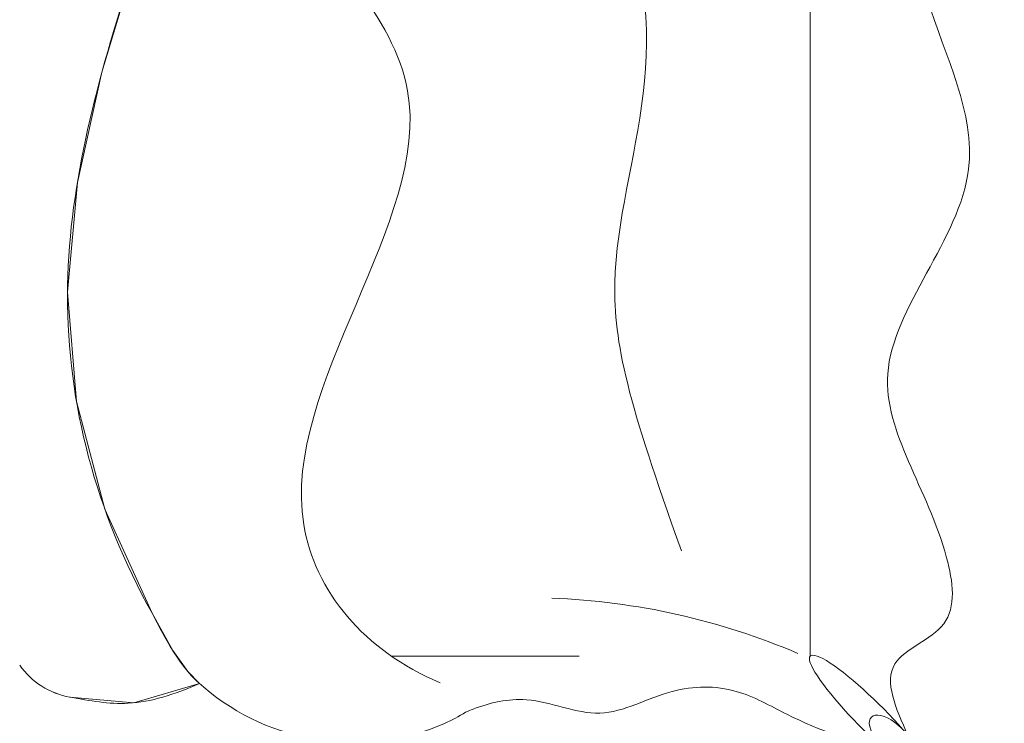
# Model space of a CAD drawing. Units: inches. Extents: x 2083 to 3317, y 1141 to 2115.
# Tile 9 of 256: x 2278 to 2324, y 1296 to 1329. Entities that reach past the tile are written whole.
import ezdxf

# ---------------------------------------------------------------- set-up
doc = ezdxf.new("R2010")
doc.units = ezdxf.units.IN
for name, color, linetype, lineweight in [('A-ANNO-DIMS', 2, 'Continuous', 18), ('A-FURN', 8, 'Continuous', 18), ('www.cadblocksfree.com', 7, 'Continuous', 9)]:
    doc.layers.add(name, color=color, linetype=linetype, lineweight=lineweight)
doc.layers.add('A-WALL-PATT', color=251, linetype='Continuous', lineweight=13, true_color=0x636466)
doc.styles.get("Standard").update_dxf_attribs({"font": 'arial.ttf'})
doc.dimstyles.new('ISO-25', dxfattribs={"dimtxt": 12, "dimasz": 12, "dimexe": 1.25, "dimexo": 0.625, "dimtad": 1, "dimlunit": 3, "dimtxsty": 'Standard', "dimcen": 2.5, "dimadec": 0, "dimazin": 0, "dimtfac": 1, "dimtmove": 0, "dimatfit": 3, "dimfxl": 1, "dimarcsym": 0})

# ---------------------------------------------------------------- blocks, each defined once
blk = doc.blocks.new('bed')
at = {"layer": 'www.cadblocksfree.com', "ltscale": 0.2}
for p, q in [((3363.387, 1412.3), (3363.387, 1402.937)), ((3363.387, 1391.414), (3426.379, 1391.414))]:
    blk.add_line(p, q, dxfattribs=at)
for centre, radius, start, end in [((3365.21, 1427.605), 3.937, 125.4209, 169.6982), ((3370.55, 1414.186), 11.465, 139.4648, 203.3712), ((3367.278, 1412.869), 7.939, 204.0179, 212.619), ((3331.909, 1405.558), 34.378, 336.8495, 357.9003)]:
    blk.add_arc(centre, radius, start, end, dxfattribs=at)
at = {"layer": 'www.cadblocksfree.com', "ltscale": 0.2, "extrusion": (0, 0, -1)}
for centre, major_axis, ratio, start_param, end_param in [((3360.344, 1388.371), (3.043, 3.043), 0.168252, 4.250342, 8.316029), ((3359.289, 1387.316), (1.055, 1.055), 0.453532, 4.422107, 8.144264)]:
    blk.add_ellipse(centre, major_axis=major_axis, ratio=ratio, start_param=start_param, end_param=end_param, dxfattribs=at)
at = {"layer": 'www.cadblocksfree.com', "ltscale": 0.2}
for points, knots in [([(3365.512, 1424.213), (3370.519, 1427.004), (3381.149, 1429.825), (3396.214, 1425.866), (3410.541, 1420.654), (3420.273, 1432.695), (3425.882, 1426.771), (3428.534, 1423.97)], [0.099185, 0.099185, 0.099185, 0.099185, 0.523647, 0.927087, 1.289918, 1.564439, 1.810555, 1.810555, 1.810555, 1.810555]), ([(3361.336, 1428.309), (3361.334, 1428.297), (3361.16, 1427.338), (3360.778, 1425.173), (3361.469, 1423.14), (3362.014, 1421.845)], [0.3128349, 0.3128349, 0.3128349, 0.3128349, 0.313751, 0.386958, 0.4759027, 0.4759027, 0.4759027, 0.4759027]), ([(3362.057, 1409.866), (3363.638, 1413.65), (3372.978, 1421.337), (3389.682, 1406.045), (3402.396, 1419.984), (3416.037, 1420.167), (3423.233, 1415.231), (3427.827, 1408.899)], [0.029901, 0.029901, 0.029901, 0.029901, 0.276967, 0.797115, 1.093669, 1.464666, 1.788489, 1.788489, 1.788489, 1.788489]), ([(3368.632, 1397.839), (3375.978, 1400.489), (3385.349, 1402.757), (3397.531, 1395.273), (3413.593, 1410.377), (3407.806, 1395.019), (3420.759, 1398.2)], [0.029901, 0.029901, 0.029901, 0.029901, 0.276967, 0.797115, 1.093669, 1.16836, 1.16836, 1.16836, 1.16836]), ([(3358.529, 1387.473), (3359.098, 1389.205), (3359.955, 1391.816), (3361.924, 1395.149), (3361.896, 1398.555), (3359.883, 1401.841), (3361.557, 1405.208), (3361.034, 1407.507), (3360.643, 1408.467), (3360.591, 1408.59)], [0, 0, 0, 0, 0.138875, 0.2092702, 0.2901949, 0.3858479, 0.4804923, 0.5489252, 0.5590752, 0.5590752, 0.5590752, 0.5590752]), ([(3430.32, 1386.556), (3427.327, 1387.653), (3422.148, 1389.55), (3414.529, 1384.137), (3405.607, 1387.046), (3396.29, 1386.314), (3386.838, 1381.282), (3377.742, 1390.272), (3370.778, 1384.799), (3364.626, 1383.966), (3363.275, 1388.265), (3360.778, 1387.151), (3359.446, 1386.556)], [0, 0, 0, 0, 8.93042, 15.449194, 25.485629, 34.878505, 43.598887, 54.554403, 64.16647, 67.461673, 70.610457, 74.213583, 74.213583, 74.213583, 74.213583])]:
    blk.add_open_spline(points, degree=3, knots=knots, dxfattribs=at)
for points in [[(3361.235, 1424.042), (3361.236, 1424.042), (3361.237, 1424.043), (3361.239, 1424.043)], [(3361.837, 1421.637), (3362.352, 1422.25), (3362.867, 1422.863), (3365.512, 1424.213)]]:
    blk.add_open_spline(points, degree=3, dxfattribs=at)
blk = doc.blocks.new('*D23')
at = {"layer": 'A-ANNO-DIMS', "color": 0, "lineweight": -2, "transparency": 16777216}
for p, q in [((2335.205, 1362.114), (2335.205, 1476.472)), ((2322.885, 1362.114), (2336.455, 1362.114)), ((2335.205, 1306.473), (2335.205, 1350.114)), ((2322.885, 1294.473), (2336.455, 1294.473))]:
    blk.add_line(p, q, dxfattribs=at)
at = {"layer": 'A-ANNO-DIMS', "color": 0, "transparency": 16777216}
for points in [[(2333.205, 1350.114), (2337.205, 1350.114), (2335.205, 1362.114)], [(2333.205, 1306.473), (2337.205, 1306.473), (2335.205, 1294.473)]]:
    blk.add_solid(points, dxfattribs=at)
at = {"layer": 'Defpoints', "color": 0, "transparency": 16777216}
for p in [(2322.26, 1362.114), (2335.205, 1362.114), (2322.26, 1294.473)]:
    blk.add_point(p, dxfattribs=at)
at = {"layer": 'A-ANNO-DIMS', "color": 0, "transparency": 16777216, "insert": (2328.376, 1425.293), "char_height": 12, "attachment_point": 5, "rotation": 90}
blk.add_mtext('5\'-7 1/2" TYP.', dxfattribs=at)

msp = doc.modelspace()

# ---------------------------------------------------------------- hatches: boundary and pattern name
at = {"layer": 'A-WALL-PATT'}
h = msp.add_hatch(color=256, dxfattribs=at)
h.dxf.hatch_style = 1
h.paths.add_polyline_path([(3126.96, 2020.761), (2748.96, 2020.761), (2604.96, 2020.761), (2226.96, 2020.761), (2226.96, 1702.761), (2466.96, 1702.761), (2466.96, 1582.761), (2418.96, 1582.761), (2418.96, 1477.761), (2226.96, 1477.761), (2226.96, 1263.261), (2544.96, 1263.261), (2544.96, 1411.761), (2604.96, 1411.761), (2685.96, 1411.761), (2685.96, 1420.761), (2604.96, 1420.761), (2604.96, 1573.761), (2604.96, 1702.761), (2604.96, 2011.761), (2748.96, 2011.761), (2748.96, 1702.761), (2862.96, 1702.761), (2862.96, 1621.761), (2871.96, 1621.761), (2871.96, 1702.761), (2883.96, 1702.761), (2883.96, 1706.939, -0.026459), (2883.96, 1711.761), (2757.96, 1711.761), (2757.96, 1807.761), (2787.96, 1807.761), (2787.96, 1812.261), (2757.96, 1812.261), (2757.96, 2011.761), (2877.96, 2011.761), (2877.96, 1812.261), (2847.96, 1812.261), (2847.96, 1807.761), (2889.836, 1807.761), (2889.836, 1812.261), (2882.46, 1812.261), (2882.46, 2011.761), (3117.96, 2011.761), (3117.96, 1812.261), (2937.836, 1812.261), (2937.836, 1807.761), (2995.71, 1807.761), (2995.71, 1796.118), (3000.21, 1796.118), (3000.21, 1807.761), (3117.96, 1807.761), (3117.96, 1711.761), (3000.21, 1711.761), (3000.21, 1760.118), (2998.573, 1760.118, -0.020711), (2995.71, 1760.118), (2995.71, 1711.761), (2931.96, 1711.761), (2931.96, 1702.761), (3126.96, 1702.761)])
h.paths.add_polyline_path([(2471.46, 2011.761), (2471.46, 1810.011), (2462.717, 1810.011), (2462.717, 1805.511), (2505.96, 1805.511), (2505.96, 1810.011), (2475.96, 1810.011), (2475.96, 2011.761), (2595.96, 2011.761), (2595.96, 1810.011), (2565.96, 1810.011), (2565.96, 1805.511), (2595.96, 1805.511), (2595.96, 1711.761), (2235.96, 1711.761), (2235.96, 1805.511), (2353.71, 1805.511), (2353.71, 1796.054), (2358.21, 1796.054), (2358.21, 1805.511), (2414.717, 1805.511), (2414.717, 1810.011), (2235.96, 1810.011), (2235.96, 2011.761)], flags=16)
h.paths.add_polyline_path([(2270.205, 1994.61), (2270.205, 1970.61), (2246.205, 1970.61), (2246.205, 1994.61)], flags=0)
edge = h.paths.add_edge_path(flags=0)
edge.add_ellipse((2332.027, 1899.798), major_axis=(-3.043, 3.043), ratio=0.168252, start_angle=-161.3322, end_angle=-156.3071, ccw=False)
edge.add_ellipse((2333.082, 1898.744), major_axis=(-1.055, 1.055), ratio=0.453532, start_angle=-123.371, end_angle=-94.1591)
edge = h.paths.add_edge_path(flags=0)
edge.add_ellipse((2332.027, 1968.876), major_axis=(3.043, 3.043), ratio=0.168252, start_angle=18.6678, end_angle=23.6929)
edge.add_spline(control_points=[(2332.926, 1970.691), (2332.227, 1970.336), (2330.894, 1969.659), (2328.413, 1970.932), (2327.204, 1967.749), (2324.71, 1969.956), (2322.533, 1967.012), (2320.013, 1971.296), (2317.68, 1968.158), (2316.041, 1967.102), (2315.427, 1966.81)], knot_values=[0, 0, 0, 0, 2.267059, 4.324559, 6.685584, 8.878641, 11.121502, 14.300359, 17.755284, 19.732645, 19.732645, 19.732645, 19.732645], degree=3, periodic=0)
edge.add_ellipse((2332.027, 1968.876), major_axis=(3.043, 3.043), ratio=0.168252, start_angle=18.6678, end_angle=23.6929, ccw=False)
edge.add_ellipse((2333.082, 1969.931), major_axis=(1.055, 1.055), ratio=0.453532, start_angle=56.629, end_angle=85.8409, ccw=False)
edge = h.paths.add_edge_path(flags=0)
edge.add_spline(control_points=[(2296.428, 1967.988), (2293.628, 1965.336), (2287.704, 1959.727), (2299.744, 1949.996), (2294.533, 1935.669), (2290.573, 1920.604), (2293.394, 1909.974), (2296.185, 1904.967)], knot_values=[0.099185, 0.099185, 0.099185, 0.099185, 0.345301, 0.619822, 0.982653, 1.386093, 1.810555, 1.810555, 1.810555, 1.810555], degree=3, periodic=0)
edge.add_spline(control_points=[(2296.185, 1904.967), (2297.384, 1902.619), (2298.001, 1901.949), (2298.553, 1901.468)], knot_values=[0.006246, 0.006246, 0.006246, 0.006246, 0.055476, 0.055476, 0.055476, 0.055476], degree=3, periodic=0)
edge.add_spline(control_points=[(2298.553, 1901.468), (2297.259, 1900.923), (2295.225, 1900.232), (2293.06, 1900.614), (2292.101, 1900.788), (2292.09, 1900.791)], knot_values=[0.312835, 0.312835, 0.312835, 0.312835, 0.40178, 0.474987, 0.475903, 0.475903, 0.475903, 0.475903], degree=3, periodic=0)
edge.add_arc((2292.794, 1904.664), 3.937, 215.4209, 259.6982, ccw=False)
edge.add_spline(control_points=[(2289.585, 1902.382), (2289.477, 1902.535), (2289.368, 1902.688), (2289.261, 1902.841)], knot_values=[0.102872, 0.102872, 0.102872, 0.102872, 0.116896, 0.116896, 0.116896, 0.116896], degree=3, periodic=0)
edge.add_spline(control_points=[(2289.261, 1902.841), (2288.687, 1902.55), (2287.64, 1902.02), (2285.881, 1901.874), (2283.853, 1901.504), (2281.72, 1899.711), (2278.467, 1899.493), (2276.157, 1901.883), (2272.259, 1899.804), (2267.778, 1901.843), (2262.244, 1900.184), (2257.415, 1901.782), (2254.318, 1900.726), (2253.178, 1900.337)], knot_values=[0, 0, 0, 0, 1.907977, 3.477176, 5.261074, 7.972851, 11.680248, 13.717921, 16.939592, 22.789562, 27.502503, 33.595215, 37.145618, 37.145618, 37.145618, 37.145618], degree=3, periodic=0)
edge.add_line((2253.178, 1900.337), (2250.244, 1902.841))
edge.add_line((2250.244, 1902.841), (2250.244, 1965.833))
edge.add_line((2250.244, 1965.833), (2253.178, 1968.337))
edge.add_spline(control_points=[(2253.178, 1968.337), (2254.318, 1967.948), (2257.415, 1966.892), (2262.244, 1968.49), (2267.778, 1966.831), (2271.527, 1968.537), (2273.876, 1967.828), (2274.207, 1967.728)], knot_values=[0, 0, 0, 0, 0.09018, 0.244935, 0.364644, 0.513233, 0.537855, 0.537855, 0.537855, 0.537855], degree=3, periodic=0)
edge.add_arc((2274.353, 1963.793), 3.937, 72.0511, 92.1279, ccw=False)
edge.add_arc((2281.297, 1985.23), 18.596, 252.0511, 288.5657)
edge.add_arc((2292.317, 1956.029), 12.646, 71.0268, 113.7782, ccw=False)
edge = h.paths.add_edge_path(flags=0)
edge.add_spline(control_points=[(2274.899, 1951.856), (2275.066, 1951.617), (2275.233, 1951.377), (2275.398, 1951.136)], knot_values=[1.409916, 1.409916, 1.409916, 1.409916, 1.43159, 1.43159, 1.43159, 1.43159], degree=3, periodic=0)
edge.add_spline(control_points=[(2275.398, 1951.136), (2275.792, 1950.562), (2276.179, 1949.984), (2276.546, 1949.397)], knot_values=[1.358238, 1.358238, 1.358238, 1.358238, 1.409916, 1.409916, 1.409916, 1.409916], degree=3, periodic=0)
edge.add_line((2276.546, 1949.397), (2277.437, 1947.862))
edge.add_spline(control_points=[(2277.437, 1947.862), (2276.304, 1945.673), (2274.64, 1942.427), (2274.632, 1938.094), (2272.799, 1930.852), (2274.356, 1943.897), (2275.948, 1947.923), (2276.546, 1949.397)], knot_values=[0.005632, 0.005632, 0.005632, 0.005632, 0.186014, 0.266002, 0.357087, 0.59639, 0.739732, 0.739732, 0.739732, 0.739732], degree=3, periodic=0)
edge.add_spline(control_points=[(2276.546, 1949.397), (2276.179, 1949.984), (2275.792, 1950.562), (2275.398, 1951.136)], knot_values=[1.358238, 1.358238, 1.358238, 1.358238, 1.409916, 1.409916, 1.409916, 1.409916], degree=3, periodic=0)
edge.add_spline(control_points=[(2275.398, 1951.136), (2274.943, 1950.08), (2274.208, 1948.025), (2273.935, 1944.851), (2272.469, 1937.627), (2273.466, 1945.696), (2274.701, 1951.059), (2274.899, 1951.856)], knot_values=[0.104364, 0.104364, 0.104364, 0.104364, 0.189636, 0.269624, 0.36071, 0.600013, 0.644622, 0.644622, 0.644622, 0.644622], degree=3, periodic=0)
h.paths.add_polyline_path([(2269.168, 1963.128, -0.357527), (2268.171, 1960.976, -0.092561), (2268.171, 1939.436, -0.357527), (2269.168, 1937.285, -0.357527), (2267.016, 1938.282, -0.164785), (2254.686, 1938.282, -0.357527), (2252.534, 1937.285, -0.357527), (2253.531, 1939.436, -0.092561), (2253.531, 1960.976, -0.357527), (2252.534, 1963.128, -0.357527), (2254.686, 1962.131, -0.164785), (2267.016, 1962.131, -0.357527)], flags=0)
h.paths.add_polyline_path([(2248.874, 1967.802), (2248.874, 1957.028), (2249.458, 1957.028), (2249.458, 1911.647), (2248.874, 1911.647), (2248.874, 1900.873), (2246.512, 1900.873, 0.197327), (2244.15, 1902.457), (2244.15, 1966.218, 0.197327), (2246.512, 1967.802)], flags=0)
h.paths.add_polyline_path([(2269.168, 1931.389, -0.357527), (2268.171, 1929.238, -0.092561), (2268.171, 1907.698, -0.357527), (2269.168, 1905.547, -0.357527), (2267.016, 1906.544, -0.164785), (2254.686, 1906.544, -0.357527), (2252.534, 1905.547, -0.357527), (2253.531, 1907.698, -0.092561), (2253.531, 1929.238, -0.357527), (2252.534, 1931.389, -0.357527), (2254.686, 1930.392, -0.164785), (2267.016, 1930.392, -0.357527)], flags=0)
edge = h.paths.add_edge_path(flags=0)
edge.add_spline(control_points=[(2276.197, 1906.724), (2276.168, 1909.029), (2276.114, 1913.372), (2270.598, 1924.925), (2273.905, 1919.013), (2275.922, 1916.262), (2275.475, 1912.402), (2277.258, 1910.381), (2276.696, 1908.225), (2276.646, 1906.813), (2276.618, 1906.008)], knot_values=[0, 0, 0, 0, 8.61026, 16.221274, 18.843057, 23.804898, 27.440828, 29.356102, 31.203478, 33.650687, 33.650687, 33.650687, 33.650687], degree=3, periodic=0)
edge.add_spline(control_points=[(2276.618, 1906.008), (2276.623, 1905.624), (2276.498, 1904.629), (2275.442, 1903.855), (2274.937, 1903.08), (2274.859, 1902.841)], knot_values=[0.156488, 0.156488, 0.156488, 0.156488, 0.184398, 0.231376, 0.250598, 0.250598, 0.250598, 0.250598], degree=3, periodic=0)
edge.add_line((2274.859, 1902.841), (2276.506, 1902.841))
edge.add_spline(control_points=[(2276.506, 1902.841), (2276.788, 1903.085), (2277.665, 1904.125), (2278.25, 1904.341), (2277.654, 1908.527), (2278.156, 1906.228), (2278.1, 1905.286), (2278.847, 1904.069), (2277.857, 1903.415), (2277.874, 1902.991), (2277.904, 1902.841)], knot_values=[0.059574, 0.059574, 0.059574, 0.059574, 0.080753, 0.103741, 0.16972, 0.176036, 0.207137, 0.240474, 0.262341, 0.27366, 0.27366, 0.27366, 0.27366], degree=3, periodic=0)
edge.add_line((2277.904, 1902.841), (2280.03, 1902.841))
edge.add_spline(control_points=[(2280.03, 1902.841), (2279.888, 1903.088), (2279.499, 1903.982), (2280.152, 1905.939), (2278.104, 1909.658), (2279.762, 1907.185), (2280.328, 1904.875), (2280.485, 1903.49), (2281.463, 1903.249), (2281.758, 1902.936), (2281.834, 1902.841)], knot_values=[0.013856, 0.013856, 0.013856, 0.013856, 0.034874, 0.088867, 0.107879, 0.126738, 0.158714, 0.193757, 0.217487, 0.226722, 0.226722, 0.226722, 0.226722], degree=3, periodic=0)
edge.add_spline(control_points=[(2281.834, 1902.841), (2281.788, 1902.827), (2281.647, 1902.783), (2281.396, 1902.859), (2281.088, 1902.985), (2280.721, 1903.061), (2280.333, 1903.026), (2280.125, 1902.899), (2280.03, 1902.841)], knot_values=[0, 0, 0, 0, 0.14413, 0.435517, 0.749276, 1.153046, 1.548371, 1.878348, 1.878348, 1.878348, 1.878348], degree=3, periodic=0)
edge.add_line((2280.03, 1902.841), (2277.904, 1902.841))
edge.add_spline(control_points=[(2277.904, 1902.841), (2277.893, 1902.796), (2277.865, 1902.68), (2277.607, 1902.687), (2277.274, 1902.801), (2276.838, 1902.62), (2276.584, 1902.789), (2276.506, 1902.841)], knot_values=[0, 0, 0, 0, 0.127189, 0.326199, 0.628009, 1.24357, 1.515331, 1.515331, 1.515331, 1.515331], degree=3, periodic=0)
edge.add_line((2276.506, 1902.841), (2274.859, 1902.841))
edge.add_spline(control_points=[(2274.859, 1902.841), (2274.814, 1902.899), (2274.725, 1903.013), (2274.493, 1903.119), (2274.244, 1902.961), (2273.937, 1903.185), (2273.614, 1902.983), (2273.408, 1902.883), (2273.322, 1902.841)], knot_values=[0, 0, 0, 0, 0.21843, 0.436957, 0.687977, 0.990379, 1.398396, 1.69185, 1.69185, 1.69185, 1.69185], degree=3, periodic=0)
edge.add_spline(control_points=[(2273.322, 1902.841), (2273.617, 1903.446), (2274.274, 1904.538), (2276.027, 1904.574), (2276.207, 1906.584), (2276.197, 1906.724)], knot_values=[0.012227, 0.012227, 0.012227, 0.012227, 0.059472, 0.106218, 0.134458, 0.134458, 0.134458, 0.134458], degree=3, periodic=0)
h.paths.add_polyline_path([(2270.776, 1897.79), (2270.776, 1873.79), (2246.776, 1873.79), (2246.776, 1897.79)], flags=0)
h.paths.add_polyline_path([(2353.71, 1760.005), (2353.71, 1760.054), (2358.21, 1760.054, -0.033729)], flags=0)
h.paths.add_polyline_path([(2321.819, 1737.529), (2341.995, 1737.529, -0.414214), (2343.203, 1736.321), (2343.203, 1721.021, -0.414214), (2341.995, 1719.813), (2321.819, 1719.813, -0.414214), (2320.611, 1721.021), (2320.611, 1736.321, -0.414214)], flags=0)
h.paths.add_polyline_path([(2324.235, 1736.321), (2339.579, 1736.321, -0.414214), (2341.995, 1733.905), (2341.995, 1725.45, -0.414214), (2339.579, 1723.034), (2333.681, 1723.034), (2333.845, 1722.045, -0.870646), (2335.425, 1721.826, -0.767327), (2333.923, 1721.423), (2331.291, 1721.423, -0.767327), (2329.788, 1721.826, -0.870646), (2331.368, 1722.045), (2331.533, 1723.034), (2324.235, 1723.034, -0.414214), (2321.819, 1725.45), (2321.819, 1733.905, -0.414214)], flags=0)
h.paths.add_polyline_path([(2570.484, 1928.615), (2589.684, 1928.615), (2590.169, 1928.615), (2590.169, 1904.993), (2570.484, 1904.993)], flags=0)
h.paths.add_polyline_path([(2574.447, 1927.264, -1), (2572.829, 1927.264, -1)], flags=0)
h.paths.add_polyline_path([(2573.09, 1926.941), (2573.925, 1927.776), (2574.148, 1927.553), (2573.313, 1926.718)], flags=0)
h.paths.add_polyline_path([(2578.779, 1919.73, -1), (2571.592, 1919.73, -1)], flags=0)
h.paths.add_polyline_path([(2578.385, 1919.73, -1), (2571.985, 1919.73, -1)], flags=0)
h.paths.add_polyline_path([(2331.596, 1729.476, -1), (2333.618, 1729.476, -1)], flags=0)
h.paths.add_polyline_path([(2578.034, 1927.264, -1), (2576.416, 1927.264, -1)], flags=0)
h.paths.add_polyline_path([(2576.689, 1927.531), (2576.912, 1927.754), (2577.747, 1926.919), (2577.524, 1926.696)], flags=0)
h.paths.add_polyline_path([(2578.139, 1909.86, -1), (2572.232, 1909.86, -1)], flags=0)
h.paths.add_polyline_path([(2577.745, 1909.86, -1), (2572.625, 1909.86, -1)], flags=0)
h.paths.add_polyline_path([(2583.798, 1927.264, -1), (2582.179, 1927.264, -1)], flags=0)
h.paths.add_polyline_path([(2582.719, 1927.754), (2583.554, 1926.919), (2583.331, 1926.696), (2582.496, 1927.531)], flags=0)
h.paths.add_polyline_path([(2582.496, 1927.531), (2582.719, 1927.754), (2583.554, 1926.919), (2583.331, 1926.696)], flags=0)
h.paths.add_polyline_path([(2587.739, 1920.53, -1), (2581.832, 1920.53, -1)], flags=0)
h.paths.add_polyline_path([(2587.345, 1920.53, -1), (2582.225, 1920.53, -1)], flags=0)
h.paths.add_polyline_path([(2587.385, 1927.264, -1), (2585.766, 1927.264, -1)], flags=0)
h.paths.add_polyline_path([(2586.082, 1926.98), (2586.917, 1927.815), (2587.14, 1927.593), (2586.305, 1926.758)], flags=0)
h.paths.add_polyline_path([(2588.379, 1910.66, -1), (2581.192, 1910.66, -1)], flags=0)
h.paths.add_polyline_path([(2587.985, 1910.66, -1), (2581.585, 1910.66, -1)], flags=0)
h.paths.add_polyline_path([(2417.168, 1729.478), (2437.344, 1729.478, -0.414214), (2438.552, 1728.27), (2438.552, 1712.969, -0.414214), (2437.344, 1711.761), (2417.168, 1711.761, -0.414214), (2415.96, 1712.969), (2415.96, 1728.27, -0.414214)], flags=0)
h.paths.add_polyline_path([(2419.584, 1728.27), (2434.928, 1728.27, -0.414214), (2437.344, 1725.854), (2437.344, 1717.398, -0.414214), (2434.928, 1714.983), (2429.029, 1714.983), (2429.194, 1713.994, -0.870646), (2430.774, 1713.775, -0.767327), (2429.271, 1713.372), (2426.64, 1713.372, -0.767327), (2425.137, 1713.775, -0.870646), (2426.717, 1713.994), (2426.882, 1714.983), (2419.584, 1714.983, -0.414214), (2417.168, 1717.398), (2417.168, 1725.854, -0.414214)], flags=0)
h.paths.add_polyline_path([(2419.584, 1728.27), (2434.928, 1728.27, -0.414214), (2437.344, 1725.854), (2437.344, 1717.398, -0.414214), (2434.928, 1714.983), (2429.029, 1714.983), (2428.358, 1719.009), (2427.553, 1719.009), (2426.882, 1714.983), (2419.584, 1714.983, -0.414214), (2417.168, 1717.398), (2417.168, 1725.854, -0.414214)], flags=0)
h.paths.add_polyline_path([(2426.944, 1721.425, -1), (2428.967, 1721.425, -1)], flags=0)
h.paths.add_polyline_path([(2475.96, 1702.761), (2595.96, 1702.761), (2595.96, 1582.761), (2475.96, 1582.761)], flags=16)
h.paths.add_polyline_path([(2427.96, 1573.761), (2595.96, 1573.761), (2595.96, 1468.761), (2595.96, 1420.761), (2384.46, 1420.761), (2384.46, 1468.761), (2427.96, 1468.761)], flags=16)
h.paths.add_polyline_path([(2379.96, 1468.761), (2379.96, 1420.761), (2235.96, 1420.761), (2235.96, 1468.761)], flags=16)
h.paths.add_polyline_path([(2317.816, 1466.696), (2337.992, 1466.696, -0.414214), (2339.2, 1465.488), (2339.2, 1450.187, -0.414214), (2337.992, 1448.979), (2317.816, 1448.979, -0.414214), (2316.608, 1450.187), (2316.608, 1465.488, -0.414214)], flags=0)
h.paths.add_polyline_path([(2320.232, 1465.488), (2335.576, 1465.488, -0.414214), (2337.992, 1463.072), (2337.992, 1454.616, -0.414214), (2335.576, 1452.2), (2329.677, 1452.2), (2329.842, 1451.212, -0.870646), (2331.422, 1450.992, -0.767327), (2329.92, 1450.59), (2327.288, 1450.59, -0.767327), (2325.785, 1450.992, -0.870646), (2327.365, 1451.212), (2327.53, 1452.2), (2320.232, 1452.2, -0.414214), (2317.816, 1454.616), (2317.816, 1463.072, -0.414214)], flags=0)
h.paths.add_polyline_path([(2320.232, 1465.488), (2335.576, 1465.488, -0.414214), (2337.992, 1463.072), (2337.992, 1454.616, -0.414214), (2335.576, 1452.2), (2329.677, 1452.2), (2329.006, 1456.227), (2328.201, 1456.227), (2327.53, 1452.2), (2320.232, 1452.2, -0.414214), (2317.816, 1454.616), (2317.816, 1463.072, -0.414214)], flags=0)
h.paths.add_polyline_path([(2327.593, 1458.643, -1), (2329.615, 1458.643, -1)], flags=0)
h.paths.add_polyline_path([(2244.412, 1433.34), (2241.921, 1433.34, -0.414214), (2240.018, 1435.244), (2240.018, 1440.953, -0.414211), (2241.921, 1442.856), (2244.412, 1442.856, -1.976472)], flags=0)
h.paths.add_polyline_path([(2245.357, 1434.398, -0.414214), (2245.357, 1441.799, -2.144098)], flags=0)
h.paths.add_polyline_path([(2535.96, 1416.261), (2535.96, 1272.261), (2235.96, 1272.261), (2235.96, 1416.261)], flags=16)
h.paths.add_polyline_path([(2260.12, 1384.293), (2260.12, 1362.039), (2237.865, 1362.039), (2237.865, 1384.293)], flags=0)
edge = h.paths.add_edge_path(flags=0)
edge.add_line((2318.252, 1362.093), (2318.146, 1362.001))
edge.add_ellipse((2317.445, 1360.431), major_axis=(2.822, 2.822), ratio=0.168252, start_angle=18.6678, end_angle=20.9481, ccw=False)
edge.add_ellipse((2318.423, 1361.409), major_axis=(0.978, 0.978), ratio=0.453532, start_angle=56.629, end_angle=70.2262, ccw=False)
edge = h.paths.add_edge_path(flags=0)
edge.add_line((2319.107, 1295.571), (2319.015, 1295.677))
edge.add_ellipse((2317.445, 1296.378), major_axis=(-2.822, 2.822), ratio=0.168252, start_angle=-161.3322, end_angle=-159.0519, ccw=False)
edge.add_ellipse((2318.423, 1295.4), major_axis=(-0.978, 0.978), ratio=0.453532, start_angle=-123.371, end_angle=-109.7738)
edge = h.paths.add_edge_path(flags=0)
edge.add_spline(control_points=[(2284.21, 1301.17), (2284.581, 1300.445), (2284.891, 1299.892), (2285.16, 1299.461)], knot_values=[0.039066, 0.039066, 0.039066, 0.039066, 0.055476, 0.055476, 0.055476, 0.055476], degree=3, periodic=0)
edge.add_line((2285.16, 1299.461), (2284.21, 1301.17))
edge = h.paths.add_edge_path(flags=0)
edge.add_line((2280.412, 1297.298), (2283.37, 1297.036))
edge.add_line((2283.37, 1297.036), (2286.406, 1297.926))
edge.add_spline(control_points=[(2286.406, 1297.926), (2285.305, 1297.463), (2284.345, 1297.129), (2283.37, 1297.036)], knot_values=[0.394369, 0.394369, 0.394369, 0.394369, 0.475903, 0.475903, 0.475903, 0.475903], degree=3, periodic=0)
edge.add_spline(control_points=[(2283.37, 1297.036), (2283.281, 1297.028), (2282.316, 1296.957), (2281.313, 1297.134), (2280.423, 1297.296), (2280.412, 1297.298)], knot_values=[0.312835, 0.312835, 0.312835, 0.312835, 0.320246, 0.393453, 0.394369, 0.394369, 0.394369, 0.394369], degree=3, periodic=0)
edge = h.paths.add_edge_path(flags=0)
edge.add_line((2284.436, 1359.607), (2280.446, 1355.328))
edge.add_line((2280.446, 1355.328), (2279.58, 1351.018))
edge.add_line((2279.58, 1351.018), (2282.413, 1346.58))
edge.add_spline(control_points=[(2282.413, 1346.58), (2283.153, 1345.589), (2284.253, 1344.029), (2284.801, 1342.387), (2284.935, 1341.806)], knot_values=[1.240098, 1.240098, 1.240098, 1.240098, 1.332892, 1.382712, 1.382712, 1.382712, 1.382712], degree=3, periodic=0)
edge.add_spline(control_points=[(2284.935, 1341.806), (2285.319, 1340.141), (2285.233, 1338.409), (2284.91, 1336.654)], knot_values=[1.097484, 1.097484, 1.097484, 1.097484, 1.240098, 1.240098, 1.240098, 1.240098], degree=3, periodic=0)
edge.add_spline(control_points=[(2284.91, 1336.654), (2284.587, 1334.899), (2284.027, 1333.12), (2283.463, 1331.361)], knot_values=[0.95487, 0.95487, 0.95487, 0.95487, 1.097484, 1.097484, 1.097484, 1.097484], degree=3, periodic=0)
edge.add_line((2283.463, 1331.361), (2281.89, 1326.153))
edge.add_line((2281.89, 1326.153), (2280.756, 1321.056))
edge.add_line((2280.756, 1321.056), (2280.299, 1316.002))
edge.add_line((2280.299, 1316.002), (2280.716, 1310.95))
edge.add_line((2280.716, 1310.95), (2282.028, 1305.972))
edge.add_line((2282.028, 1305.972), (2284.21, 1301.17))
edge.add_spline(control_points=[(2284.21, 1301.17), (2283.341, 1302.73), (2282.612, 1304.336), (2282.028, 1305.972)], knot_values=[0.099185, 0.099185, 0.099185, 0.099185, 0.241799, 0.241799, 0.241799, 0.241799], degree=3, periodic=0)
edge.add_spline(control_points=[(2282.028, 1305.972), (2281.444, 1307.608), (2281.005, 1309.273), (2280.716, 1310.95)], knot_values=[0.241799, 0.241799, 0.241799, 0.241799, 0.384413, 0.384413, 0.384413, 0.384413], degree=3, periodic=0)
edge.add_spline(control_points=[(2280.716, 1310.95), (2280.433, 1312.588), (2280.289, 1314.277), (2280.299, 1315.962), (2280.299, 1316.002)], knot_values=[0.384413, 0.384413, 0.384413, 0.384413, 0.523647, 0.527028, 0.527028, 0.527028, 0.527028], degree=3, periodic=0)
edge.add_spline(control_points=[(2280.299, 1316.002), (2280.312, 1317.687), (2280.478, 1319.368), (2280.756, 1321.056)], knot_values=[0.527028, 0.527028, 0.527028, 0.527028, 0.669642, 0.669642, 0.669642, 0.669642], degree=3, periodic=0)
edge.add_spline(control_points=[(2280.756, 1321.056), (2281.035, 1322.744), (2281.426, 1324.44), (2281.89, 1326.153)], knot_values=[0.669642, 0.669642, 0.669642, 0.669642, 0.812256, 0.812256, 0.812256, 0.812256], degree=3, periodic=0)
edge.add_spline(control_points=[(2281.89, 1326.153), (2282.264, 1327.533), (2282.788, 1329.262), (2283.353, 1331.018), (2283.463, 1331.361)], knot_values=[0.812256, 0.812256, 0.812256, 0.812256, 0.927087, 0.95487, 0.95487, 0.95487, 0.95487], degree=3, periodic=0)
edge.add_line((2283.463, 1331.361), (2284.91, 1336.654))
edge.add_line((2284.91, 1336.654), (2284.935, 1341.806))
edge.add_line((2284.935, 1341.806), (2282.413, 1346.58))
edge.add_spline(control_points=[(2282.413, 1346.58), (2281.275, 1348.104), (2280.078, 1349.57), (2279.58, 1351.018)], knot_values=[1.382712, 1.382712, 1.382712, 1.382712, 1.525326, 1.525326, 1.525326, 1.525326], degree=3, periodic=0)
edge.add_spline(control_points=[(2279.58, 1351.018), (2279.443, 1351.415), (2279.136, 1352.857), (2279.735, 1354.29), (2280.446, 1355.328)], knot_values=[1.525326, 1.525326, 1.525326, 1.525326, 1.564439, 1.667941, 1.667941, 1.667941, 1.667941], degree=3, periodic=0)
edge.add_spline(control_points=[(2280.446, 1355.328), (2281.426, 1356.758), (2282.931, 1358.183), (2284.436, 1359.607)], knot_values=[1.667941, 1.667941, 1.667941, 1.667941, 1.810555, 1.810555, 1.810555, 1.810555], degree=3, periodic=0)
edge.add_arc((2280.623, 1348.518), 11.726, 71.0268, 113.7782)
edge.add_arc((2270.405, 1375.595), 17.244, 252.0511, 288.5657, ccw=False)
edge.add_arc((2263.966, 1355.718), 3.651, 72.0511, 92.1279)
edge.add_arc((2263.966, 1355.718), 3.651, 92.1279, 177.9851)
edge.add_spline(control_points=[(2260.318, 1355.846), (2260.26, 1354.221), (2260.551, 1350.187), (2262.999, 1346.766), (2264.473, 1344.649)], knot_values=[1.43159, 1.43159, 1.43159, 1.43159, 1.564144, 1.770695, 1.770695, 1.770695, 1.770695], degree=3, periodic=0)
edge.add_line((2264.473, 1344.649), (2264.936, 1343.983))
edge.add_spline(control_points=[(2263.801, 1340.248), (2263.843, 1340.514), (2264.067, 1341.756), (2264.513, 1343.002), (2264.935, 1343.981)], knot_values=[0.53657, 0.53657, 0.53657, 0.53657, 0.559349, 0.644622, 0.644622, 0.644622, 0.644622], degree=3, periodic=0)
edge.add_spline(control_points=[(2264.935, 1343.981), (2265.118, 1343.715), (2265.299, 1343.448), (2265.477, 1343.179)], knot_values=[1.384077, 1.384077, 1.384077, 1.384077, 1.409916, 1.409916, 1.409916, 1.409916], degree=3, periodic=0)
edge.add_spline(control_points=[(2265.477, 1343.179), (2265.655, 1342.911), (2265.829, 1342.641), (2265.999, 1342.369)], knot_values=[1.358238, 1.358238, 1.358238, 1.358238, 1.384077, 1.384077, 1.384077, 1.384077], degree=3, periodic=0)
edge.add_line((2265.999, 1342.369), (2266.826, 1340.946))
edge.add_spline(control_points=[(2266.826, 1340.946), (2268.894, 1337.09), (2271.398, 1325.843), (2270.516, 1310.569), (2275.919, 1301.861), (2277.79, 1299.199)], knot_values=[0.116896, 0.116896, 0.116896, 0.116896, 0.472987, 1.050969, 1.313793, 1.313793, 1.313793, 1.313793], degree=3, periodic=0)
edge.add_spline(control_points=[(2277.79, 1299.199), (2277.839, 1299.128), (2277.889, 1299.057), (2277.94, 1298.987)], knot_values=[0.109884, 0.109884, 0.109884, 0.109884, 0.116896, 0.116896, 0.116896, 0.116896], degree=3, periodic=0)
edge.add_line((2277.94, 1298.987), (2277.789, 1299.199))
edge.add_spline(control_points=[(2277.789, 1299.199), (2277.257, 1298.929), (2276.286, 1298.438), (2275.039, 1298.334), (2274.383, 1298.239), (2274.215, 1298.209)], knot_values=[33.12187, 33.12187, 33.12187, 33.12187, 35.029056, 36.598255, 37.144827, 37.144827, 37.144827, 37.144827], degree=3, periodic=0)
edge.add_line((2274.215, 1298.209), (2273.073, 1297.893))
edge.add_spline(control_points=[(2273.073, 1297.893), (2272.323, 1297.58), (2271.039, 1296.511), (2269.248, 1296.226), (2268.423, 1296.375)], knot_values=[26.532584, 26.532584, 26.532584, 26.532584, 29.198919, 31.839101, 31.839101, 31.839101, 31.839101], degree=3, periodic=0)
edge.add_line((2268.423, 1296.375), (2263.879, 1297.458))
edge.add_spline(control_points=[(2263.879, 1297.458), (2263.556, 1297.359), (2261.86, 1296.839), (2260.239, 1297.282), (2258.933, 1297.516)], knot_values=[15.919551, 15.919551, 15.919551, 15.919551, 16.939592, 21.226067, 21.226067, 21.226067, 21.226067], degree=3, periodic=0)
edge.add_line((2258.933, 1297.516), (2254.055, 1297.329))
edge.add_spline(control_points=[(2254.055, 1297.329), (2253.756, 1297.296), (2252.114, 1297.165), (2250.462, 1297.544), (2249.13, 1297.668)], knot_values=[5.306517, 5.306517, 5.306517, 5.306517, 6.276435, 10.613034, 10.613034, 10.613034, 10.613034], degree=3, periodic=0)
edge.add_line((2249.13, 1297.668), (2244.332, 1296.878))
edge.add_line((2244.332, 1296.878), (2241.611, 1299.199))
edge.add_line((2241.611, 1299.199), (2241.611, 1357.609))
edge.add_line((2241.611, 1357.609), (2244.332, 1359.931))
edge.add_line((2244.332, 1359.931), (2252.729, 1359.543))
edge.add_spline(control_points=[(2252.729, 1359.543), (2252.871, 1359.546), (2253.306, 1359.548), (2253.74, 1359.514), (2254.032, 1359.482)], knot_values=[0.233291, 0.233291, 0.233291, 0.233291, 0.244935, 0.268927, 0.268927, 0.268927, 0.268927], degree=3, periodic=0)
edge.add_line((2254.032, 1359.482), (2259.587, 1359.416))
edge.add_spline(control_points=[(2259.587, 1359.416), (2260.677, 1359.629), (2262.073, 1359.897), (2263.524, 1359.459), (2263.83, 1359.366)], knot_values=[0.422516, 0.422516, 0.422516, 0.422516, 0.513233, 0.537855, 0.537855, 0.537855, 0.537855], degree=3, periodic=0)
edge.add_arc((2263.966, 1355.718), 3.651, 72.0511, 92.1279, ccw=False)
edge.add_arc((2270.405, 1375.595), 17.244, 252.0511, 288.5657)
edge.add_arc((2280.623, 1348.518), 11.726, 71.0268, 113.7782, ccw=False)
h.paths.add_polyline_path([(2240.341, 1359.435), (2240.341, 1349.444), (2240.882, 1349.444), (2240.882, 1307.365), (2240.341, 1307.365), (2240.341, 1297.374), (2238.15, 1297.374, 0.197327), (2235.96, 1298.843), (2235.96, 1357.966, 0.197327), (2238.15, 1359.435)], flags=0)
h.paths.add_polyline_path([(2259.158, 1355.101, -0.357527), (2258.233, 1353.106, -0.092561), (2258.233, 1333.133, -0.357527), (2259.158, 1331.138, -0.357527), (2257.163, 1332.062, -0.164785), (2245.729, 1332.062, -0.357527), (2243.735, 1331.138, -0.357527), (2244.659, 1333.133, -0.092561), (2244.659, 1353.106, -0.357527), (2243.735, 1355.101, -0.357527), (2245.729, 1354.176, -0.164785), (2257.163, 1354.176, -0.357527)], flags=0)
edge = h.paths.add_edge_path(flags=0)
edge.add_line((2265.999, 1342.369), (2266.826, 1340.946))
edge.add_line((2266.826, 1340.946), (2265.308, 1337.814))
edge.add_line((2265.308, 1337.814), (2264.358, 1334.653))
edge.add_line((2264.358, 1334.653), (2264.262, 1333.8))
edge.add_spline(control_points=[(2264.262, 1333.8), (2264.208, 1333.187), (2264.162, 1332.366), (2264.007, 1331.414), (2263.969, 1331.202)], knot_values=[0.464444, 0.464444, 0.464444, 0.464444, 0.516691, 0.531608, 0.531608, 0.531608, 0.531608], degree=3, periodic=0)
edge.add_spline(control_points=[(2263.969, 1331.202), (2263.775, 1330.119), (2263.424, 1328.791), (2263.257, 1328.531), (2263.234, 1328.515)], knot_values=[0.372682, 0.372682, 0.372682, 0.372682, 0.44885, 0.464444, 0.464444, 0.464444, 0.464444], degree=3, periodic=0)
edge.add_spline(control_points=[(2263.234, 1328.515), (2263.096, 1328.42), (2263.131, 1329.301), (2263.275, 1330.616)], knot_values=[0.280919, 0.280919, 0.280919, 0.280919, 0.372682, 0.372682, 0.372682, 0.372682], degree=3, periodic=0)
edge.add_spline(control_points=[(2263.275, 1330.616), (2263.419, 1331.93), (2263.672, 1333.677), (2263.97, 1335.315)], knot_values=[0.189157, 0.189157, 0.189157, 0.189157, 0.280919, 0.280919, 0.280919, 0.280919], degree=3, periodic=0)
edge.add_spline(control_points=[(2263.97, 1335.315), (2264.1, 1336.032), (2264.419, 1337.622), (2264.755, 1338.864), (2264.947, 1339.491)], knot_values=[0.097394, 0.097394, 0.097394, 0.097394, 0.137578, 0.189157, 0.189157, 0.189157, 0.189157], degree=3, periodic=0)
edge.add_spline(control_points=[(2264.947, 1339.491), (2265.29, 1340.606), (2265.644, 1341.494), (2265.999, 1342.369)], knot_values=[0.005632, 0.005632, 0.005632, 0.005632, 0.097394, 0.097394, 0.097394, 0.097394], degree=3, periodic=0)
h.paths.add_polyline_path([(2259.158, 1325.671, -0.357527), (2258.233, 1323.676, -0.092561), (2258.233, 1303.703, -0.357527), (2259.158, 1301.708, -0.357527), (2257.163, 1302.633, -0.164785), (2245.729, 1302.633, -0.357527), (2243.735, 1301.708, -0.357527), (2244.659, 1303.703, -0.092561), (2244.659, 1323.676, -0.357527), (2243.735, 1325.671, -0.357527), (2245.729, 1324.747, -0.164785), (2257.163, 1324.747, -0.357527)], flags=0)
edge = h.paths.add_edge_path(flags=0)
edge.add_spline(control_points=[(2261.709, 1317.311), (2261.679, 1317.418), (2261.762, 1317.389), (2262.491, 1316.09), (2262.962, 1315.301)], knot_values=[14.955861, 14.955861, 14.955861, 14.955861, 16.221274, 18.694826, 18.694826, 18.694826, 18.694826], degree=3, periodic=0)
edge.add_spline(control_points=[(2262.962, 1315.301), (2262.99, 1315.254), (2263.702, 1314.067), (2264.349, 1313.127), (2264.73, 1312.164)], knot_values=[18.694826, 18.694826, 18.694826, 18.694826, 18.843057, 22.433791, 22.433791, 22.433791, 22.433791], degree=3, periodic=0)
edge.add_spline(control_points=[(2264.73, 1312.164), (2264.876, 1311.796), (2265.177, 1310.77), (2265.143, 1309.559), (2265.248, 1308.824)], knot_values=[22.433791, 22.433791, 22.433791, 22.433791, 23.804898, 26.172756, 26.172756, 26.172756, 26.172756], degree=3, periodic=0)
edge.add_line((2265.248, 1308.824), (2265.851, 1307.172))
edge.add_spline(control_points=[(2265.851, 1307.172), (2266.065, 1306.822), (2266.384, 1306.332), (2266.424, 1305.781), (2266.42, 1305.611)], knot_values=[28.062562, 28.062562, 28.062562, 28.062562, 29.356102, 29.911721, 29.911721, 29.911721, 29.911721], degree=3, periodic=0)
edge.add_spline(control_points=[(2266.42, 1305.611), (2266.416, 1305.433), (2266.394, 1305.25), (2266.365, 1305.066)], knot_values=[29.911721, 29.911721, 29.911721, 29.911721, 30.497837, 30.497837, 30.497837, 30.497837], degree=3, periodic=0)
edge.add_line((2266.365, 1305.066), (2266.066, 1302.136))
edge.add_spline(control_points=[(2266.066, 1302.136), (2266.071, 1301.78), (2265.998, 1301.2), (2265.663, 1300.759), (2265.509, 1300.586)], knot_values=[0.156488, 0.156488, 0.156488, 0.156488, 0.184398, 0.203543, 0.203543, 0.203543, 0.203543], degree=3, periodic=0)
edge.add_line((2265.509, 1300.586), (2264.435, 1299.199))
edge.add_line((2264.435, 1299.199), (2265.962, 1299.199))
edge.add_line((2265.962, 1299.199), (2267.336, 1301.175))
edge.add_line((2267.336, 1301.175), (2267.312, 1301.986))
edge.add_spline(control_points=[(2267.312, 1301.986), (2267.261, 1302.862), (2267.16, 1303.737), (2267.271, 1303.326)], knot_values=[0.126229, 0.126229, 0.126229, 0.126229, 0.166617, 0.166617, 0.166617, 0.166617], degree=3, periodic=0)
edge.add_spline(control_points=[(2267.271, 1303.326), (2267.28, 1303.294), (2267.31, 1303.175), (2267.373, 1302.884), (2267.406, 1302.683), (2267.418, 1302.601)], knot_values=[0.166617, 0.166617, 0.166617, 0.166617, 0.16972, 0.176036, 0.180765, 0.180765, 0.180765, 0.180765], degree=3, periodic=0)
edge.add_spline(control_points=[(2267.744, 1300.988), (2267.688, 1301.151), (2267.481, 1301.657), (2267.484, 1302.145), (2267.418, 1302.601)], knot_values=[0.180765, 0.180765, 0.180765, 0.180765, 0.193767, 0.220139, 0.220139, 0.220139, 0.220139], degree=3, periodic=0)
edge.add_line((2267.418, 1302.601), (2267.744, 1300.988))
edge.add_spline(control_points=[(2267.744, 1300.988), (2267.832, 1300.732), (2267.932, 1300.31), (2267.555, 1299.975), (2267.429, 1299.829)], knot_values=[0.220139, 0.220139, 0.220139, 0.220139, 0.240474, 0.25489, 0.25489, 0.25489, 0.25489], degree=3, periodic=0)
edge.add_line((2267.429, 1299.829), (2267.258, 1299.199))
edge.add_line((2267.258, 1299.199), (2269.23, 1299.199))
edge.add_spline(control_points=[(2269.23, 1299.199), (2269.099, 1299.429), (2268.843, 1300.016), (2269.012, 1300.916), (2268.947, 1301.661)], knot_values=[0.013856, 0.013856, 0.013856, 0.013856, 0.034874, 0.067073, 0.067073, 0.067073, 0.067073], degree=3, periodic=0)
edge.add_line((2268.947, 1301.661), (2268.432, 1303.603))
edge.add_spline(control_points=[(2268.432, 1303.603), (2268.176, 1304.192), (2267.596, 1305.251), (2268.041, 1304.623), (2268.251, 1304.282)], knot_values=[0.090155, 0.090155, 0.090155, 0.090155, 0.107879, 0.120289, 0.120289, 0.120289, 0.120289], degree=3, periodic=0)
edge.add_spline(control_points=[(2268.251, 1304.282), (2268.361, 1304.105), (2269.058, 1302.918), (2269.383, 1301.59), (2269.521, 1300.776), (2269.575, 1300.556)], knot_values=[0.120289, 0.120289, 0.120289, 0.120289, 0.126738, 0.158714, 0.173506, 0.173506, 0.173506, 0.173506], degree=3, periodic=0)
edge.add_line((2269.575, 1300.556), (2270.686, 1299.421))
edge.add_spline(control_points=[(2270.686, 1299.421), (2270.767, 1299.357), (2270.838, 1299.281), (2270.903, 1299.199)], knot_values=[0.21816, 0.21816, 0.21816, 0.21816, 0.226722, 0.226722, 0.226722, 0.226722], degree=3, periodic=0)
edge.add_line((2270.937, 1299.193), (2270.903, 1299.199))
edge.add_spline(control_points=[(2270.903, 1299.199), (2270.86, 1299.186), (2270.73, 1299.146), (2270.496, 1299.216), (2270.272, 1299.308), (2270.121, 1299.348), (2270.063, 1299.36)], knot_values=[0.939174, 0.939174, 0.939174, 0.939174, 1.083304, 1.374691, 1.68845, 1.878348, 1.878348, 1.878348, 1.878348], degree=3, periodic=0)
edge.add_line((2270.063, 1299.36), (2269.23, 1299.199))
edge.add_line((2269.23, 1299.199), (2267.258, 1299.199))
edge.add_spline(control_points=[(2267.258, 1299.199), (2267.248, 1299.157), (2267.223, 1299.05), (2266.984, 1299.057), (2266.809, 1299.116), (2266.677, 1299.109), (2266.637, 1299.105)], knot_values=[0.757665, 0.757665, 0.757665, 0.757665, 0.884854, 1.083864, 1.385675, 1.515331, 1.515331, 1.515331, 1.515331], degree=3, periodic=0)
edge.add_spline(control_points=[(2266.637, 1299.105), (2266.485, 1299.089), (2266.236, 1299.017), (2266.035, 1299.151), (2265.962, 1299.199)], knot_values=[0, 0, 0, 0, 0.485905, 0.757665, 0.757665, 0.757665, 0.757665], degree=3, periodic=0)
edge.add_line((2265.962, 1299.199), (2264.435, 1299.199))
edge.add_line((2264.435, 1299.199), (2263.858, 1299.367))
edge.add_spline(control_points=[(2263.858, 1299.367), (2263.819, 1299.371), (2263.78, 1299.386), (2263.74, 1299.402)], knot_values=[0.845925, 0.845925, 0.845925, 0.845925, 0.978627, 0.978627, 0.978627, 0.978627], degree=3, periodic=0)
edge.add_line((2263.722, 1299.396), (2263.01, 1299.199))
edge.add_spline(control_points=[(2263.01, 1299.199), (2263.246, 1299.683), (2263.506, 1300.128), (2263.873, 1300.408)], knot_values=[0.012227, 0.012227, 0.012227, 0.012227, 0.052971, 0.052971, 0.052971, 0.052971], degree=3, periodic=0)
edge.add_spline(control_points=[(2263.873, 1300.408), (2263.932, 1300.453), (2264.084, 1300.553), (2264.255, 1300.624), (2264.36, 1300.665)], knot_values=[0.052971, 0.052971, 0.052971, 0.052971, 0.059472, 0.069086, 0.069086, 0.069086, 0.069086], degree=3, periodic=0)
edge.add_line((2264.36, 1300.665), (2265.142, 1301.078))
edge.add_line((2265.142, 1301.078), (2265.676, 1302.8))
edge.add_line((2265.676, 1302.8), (2265.541, 1305.704))
edge.add_line((2265.541, 1305.704), (2264.803, 1309.328))
edge.add_line((2264.803, 1309.328), (2263.041, 1314.092))
edge.add_spline(control_points=[(2263.041, 1314.092), (2262.384, 1315.671), (2261.796, 1316.998), (2261.709, 1317.311)], knot_values=[11.216896, 11.216896, 11.216896, 11.216896, 14.955861, 14.955861, 14.955861, 14.955861], degree=3, periodic=0)
h.paths.add_polyline_path([(2871.96, 1416.261), (2895.91, 1416.261), (2895.91, 1420.761), (2871.96, 1420.761), (2871.96, 1501.761), (2862.96, 1501.761), (2862.96, 1420.761), (2805.96, 1420.761), (2805.96, 1411.761), (2862.96, 1411.761), (2862.96, 1263.261), (3126.96, 1263.261), (3126.96, 1411.761), (3126.96, 1486.761), (2943.96, 1486.761), (2943.96, 1477.761), (2967.86, 1477.761), (2967.86, 1420.761), (2943.91, 1420.761), (2943.91, 1416.261), (3117.96, 1416.261), (3117.96, 1420.761), (2972.36, 1420.761), (2972.36, 1477.761), (3117.96, 1477.761), (3117.96, 1420.761), (3117.96, 1272.261), (2871.96, 1272.261)], flags=0)
h.paths.add_polyline_path([(2457.126, 1485.943), (2527.603, 1485.943), (2527.603, 1537.636), (2457.126, 1537.636)], flags=8)
h.paths.add_polyline_path([(2481.005, 1609.982), (2590.766, 1609.982), (2590.766, 1682.003), (2481.005, 1682.003)], flags=8)
h.paths.add_polyline_path([(2483.085, 1729.127), (2553.562, 1729.127), (2553.562, 1780.82), (2483.085, 1780.82)], flags=8)

# ---------------------------------------------------------------- linework, layer by layer
at = {"layer": 'A-FURN'}
for p, q in [((2283.463, 1331.361), (2281.89, 1326.153)), ((2281.89, 1326.153), (2280.756, 1321.056)), ((2280.756, 1321.056), (2280.299, 1316.002)), ((2280.299, 1316.002), (2280.716, 1310.95)), ((2280.716, 1310.95), (2282.028, 1305.972)), ((2282.028, 1305.972), (2284.21, 1301.17)), ((2284.21, 1301.17), (2285.16, 1299.461)), ((2285.16, 1299.461), (2285.856, 1298.482)), ((2285.856, 1298.482), (2286.406, 1297.926)), ((2286.406, 1297.926), (2283.37, 1297.036)), ((2283.37, 1297.036), (2280.412, 1297.298))]:
    msp.add_line(p, q, dxfattribs=at)
msp.add_arc((2281.065, 1300.89), 3.651, 215.4209, 259.6982, dxfattribs=at)

# ---------------------------------------------------------------- block references
at = {"layer": 'A-FURN', "xscale": 0.9272580240292334, "yscale": 0.9272580240292334, "zscale": 0.9272580240292334, "rotation": 90}
msp.add_blockref('bed', (3604.823, -1819.528), dxfattribs=at)

# ---------------------------------------------------------------- dimensions: what is measured, and where the dimension line sits
at = {"layer": 'A-ANNO-DIMS'}
dim = msp.add_linear_dim(base=(2335.205, 1362.114), p1=(2322.26, 1294.473), p2=(2322.26, 1362.114), angle=90, text='<> TYP.', dimstyle='ISO-25', override={"dimdec": 1, "dimlfac": 1, "dimrnd": 0, "dimzin": 1, "dimdsep": 46, "dimlunit": 4, "dimfrac": 2}, dxfattribs=at)
dim.commit()
dim.dimension.update_dxf_attribs({"geometry": '*D23', "text_midpoint": (2328.376, 1425.293)})

doc.saveas('drawing.dxf')
